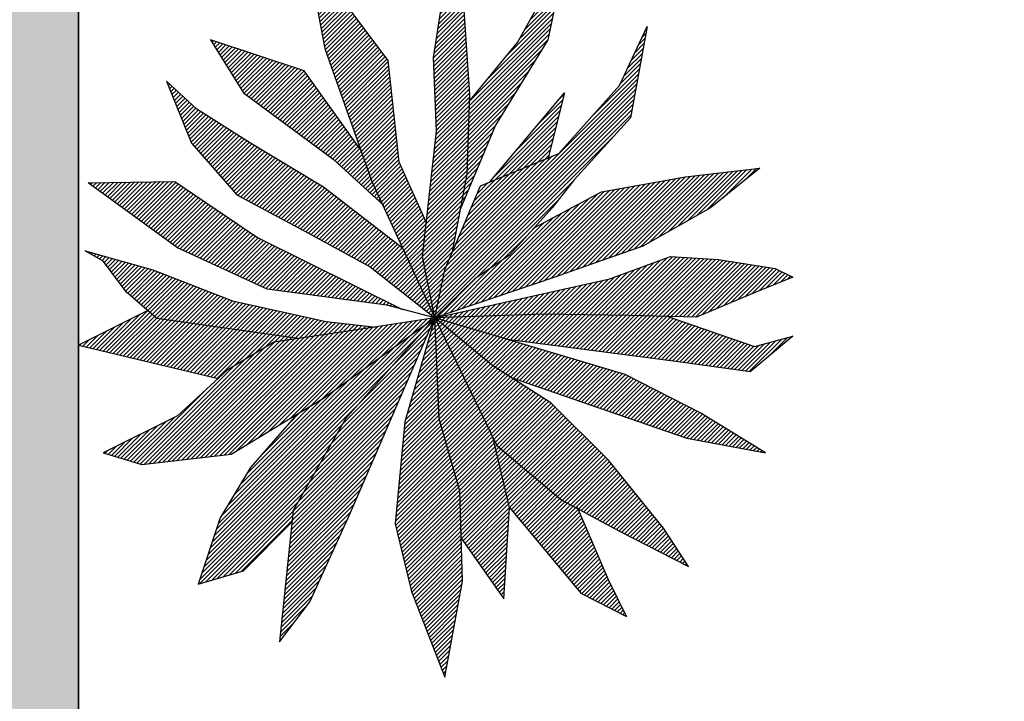
# Model space of a CAD drawing. Units: inches. Extents: x 3008 to 4088, y 1255 to 2137.
# Tile 16 of 30: x 3042 to 3093, y 1909 to 1945. Entities that reach past the tile are written whole.
import ezdxf

# ---------------------------------------------------------------- set-up
doc = ezdxf.new("R2010")
doc.units = ezdxf.units.IN
for name, color, linetype, lineweight in [('C-PROP', 1, 'Continuous', 35), ('C-PROP-PATT', 9, 'Continuous', 13), ('L-PLNT', 3, 'Continuous', 13), ('vfolhas', 114, 'Continuous', 5)]:
    doc.layers.add(name, color=color, linetype=linetype, lineweight=lineweight)
for name, color, linetype in [('vfolha', 72, 'Continuous'), ('vfolha2', 110, 'Continuous'), ('vfolhas2', 102, 'Continuous')]:
    doc.layers.add(name, color=color, linetype=linetype)
pattern_1 = [(45, (-2446.5133113, 50.986076), (-0.004419417382, 0.004419417382), [])]

# ---------------------------------------------------------------- blocks, each defined once
blk = doc.blocks.new('arbusto_PB_verde_grande')
at = {"layer": 'vfolha2'}
h = blk.add_hatch(dxfattribs=at)
h.set_pattern_fill('ANSI31', color=256, scale=0.05, style=0)
h.set_pattern_definition(pattern_1)
h.paths.add_polyline_path([(0.0294, 0.3565), (0.0003, 0.0905), (0.0263, -0.0393), (0.047, 0.0623), (0.0619, 0.0973), (0.0937, 0.2657), (0.0996, 0.4347), (0.0879, 0.6131), (0.0645, 0.7227), (0.0499, 0.6851), (0.0236, 0.5129)])
h.paths.add_polyline_path([(0.3011, 0.4379), (0.1423, 0.2487), (0.2669, 0.3002)])
h.paths.add_polyline_path([(0.38, 0.2282), (0.237, 0.1519), (0.1843, 0.0936), (0.1112, 0.0436), (0.0263, -0.0393), (0.2806, 0.0467), (0.3683, 0.078), (0.4676, 0.1124), (0.6107, 0.1938), (0.7159, 0.2782), (0.5581, 0.2595)])
h.paths.add_polyline_path([(0.561, -0.2944), (0.7275, -0.3257), (0.5902, -0.2412), (0.4296, -0.1598), (0.0263, -0.0393), (0.1492, -0.1411), (0.1884, -0.166), (0.415, -0.2444)])
h.paths.add_polyline_path([(-0.2743, -0.4478), (-0.3035, -0.7263), (-0.2392, -0.6417), (-0.1546, -0.4572), (0.0263, -0.0393), (-0.1633, -0.2538)])
h.paths.add_polyline_path([(-0.5196, -0.2474), (-0.6774, -0.3257), (-0.5956, -0.3507), (-0.4057, -0.3288), (-0.2101, -0.21), (0.0263, -0.0393), (-0.1487, -0.0659), (-0.3152, -0.091), (-0.4145, -0.1505)])
h.paths.add_polyline_path([(-0.5255, 0.2501), (-0.7095, 0.247), (-0.5196, 0.1093), (-0.3298, 0.0217), (-0.0757, -0.0128), (-0.0423, -0.0215), (-0.3502, 0.1312)])
h = blk.add_hatch(dxfattribs=at)
h.set_pattern_fill('ANSI31', color=256, scale=0.05, style=0)
h.set_pattern_definition(pattern_1)
h.paths.add_polyline_path([(-0.1896, 0.297), (-0.0855, 0.2019), (-0.1078, 0.2501), (-0.132, 0.3187), (-0.251, 0.4848), (-0.4495, 0.5505), (-0.3795, 0.4379)])
h.paths.add_polyline_path([(0.0791, -0.4071), (0.0821, -0.5063), (0.1726, -0.6355), (0.1843, -0.4415), (0.149, -0.2918), (0.0263, -0.0393), (0.0353, -0.2538)])
at = {"layer": 'vfolhas'}
h = blk.add_hatch(dxfattribs=at)
h.set_pattern_fill('ANSI31', color=256, scale=0.05, style=0)
h.set_pattern_definition(pattern_1)
h.paths.add_polyline_path([(-0.0728, 0.5067), (-0.1808, 0.6506), (-0.2334, 0.6725), (-0.2071, 0.5318), (-0.1078, 0.2501), (0.0263, -0.0393), (0.0003, 0.0905), (0.0082, 0.1624), (-0.0494, 0.2908)])
h.paths.add_polyline_path([(0.099, 0.4193), (0.0937, 0.2657), (0.0791, 0.1881), (0.1551, 0.369), (0.2661, 0.5505), (0.2836, 0.635), (0.2485, 0.6882), (0.2514, 0.635), (0.2018, 0.5443)])
h.paths.add_polyline_path([(0.1229, 0.2407), (0.047, 0.0623), (0.0263, -0.0393), (0.1112, 0.0436), (0.1843, 0.0936), (0.2748, 0.1938), (0.3215, 0.2532), (0.4413, 0.3847), (0.4763, 0.5787), (0.4179, 0.4535), (0.2894, 0.3095)])
h.paths.add_polyline_path([(0.5815, -0.0378), (0.7071, 0.0154), (0.7859, 0.0467), (0.748, 0.0655), (0.6282, 0.0842), (0.526, 0.0905), (0.3974, 0.0436), (0.0263, -0.0393), (0.2573, -0.0315), (0.4383, -0.0347)])
h.paths.add_polyline_path([(0.5202, -0.0365), (0.4383, -0.0347), (0.2573, -0.0315), (0.0263, -0.0393), (0.1796, -0.0852), (0.5377, -0.1317), (0.6954, -0.1536), (0.7859, -0.0785), (0.7041, -0.1004)])
h.paths.add_polyline_path([(0.2719, -0.2193), (0.1492, -0.1411), (0.0263, -0.0393), (0.1579, -0.3101), (0.2952, -0.4258), (0.4179, -0.4916), (0.564, -0.5667), (0.5114, -0.4853), (0.3946, -0.3414)])
h.paths.add_polyline_path([(-0.0582, -0.4759), (-0.0231, -0.6198), (0.047, -0.8013), (0.0849, -0.5979), (0.0791, -0.4071), (0.0353, -0.2538), (0.0263, -0.0393), (-0.0377, -0.26)])
h.paths.add_polyline_path([(-0.2422, 0.1405), (-0.1107, 0.0686), (0.0263, -0.0393), (-0.0423, 0.1087), (-0.2101, 0.2376), (-0.3649, 0.3314), (-0.4787, 0.4034), (-0.543, 0.4629), (-0.4904, 0.3314), (-0.3941, 0.2219)])
h = blk.add_hatch(dxfattribs=at)
h.set_pattern_fill('ANSI31', color=256, scale=0.05, style=0)
h.set_pattern_definition(pattern_1)
h.paths.add_polyline_path([(-0.5722, 0.0623), (-0.7153, 0.103), (-0.6774, 0.0811), (-0.6277, 0.0154), (-0.5635, -0.041), (-0.2646, -0.0834), (-0.1487, -0.0659), (-0.1015, -0.0588), (-0.2042, -0.0472), (-0.4028, -0.0034)])
h.paths.add_polyline_path([(-0.5635, -0.041), (-0.5828, -0.024), (-0.7299, -0.0973), (-0.4334, -0.1679), (-0.4145, -0.1505), (-0.3152, -0.091), (-0.2646, -0.0834)])
h.paths.add_polyline_path([(-0.2769, -0.4727), (-0.2743, -0.4478), (-0.1633, -0.2538), (0.0263, -0.0393), (-0.2101, -0.21), (-0.2672, -0.2447), (-0.3649, -0.357), (-0.4291, -0.4634), (-0.4759, -0.6043), (-0.3795, -0.576)])
h = blk.add_hatch(dxfattribs=at)
h.set_pattern_fill('ANSI31', color=256, scale=0.05, style=0)
h.set_pattern_definition(pattern_1)
h.paths.add_polyline_path([(0.3361, -0.623), (0.4325, -0.6731), (0.3946, -0.5948), (0.3303, -0.4446), (0.2952, -0.4258), (0.1579, -0.3101), (0.149, -0.2918), (0.1843, -0.4415)])
at = {"layer": 'vfolha'}
for p, q in [((0.0263, -0.0393), (-0.1487, -0.0659)), ((0.0263, -0.0393), (-0.0377, -0.26)), ((0.0353, -0.2538), (0.0263, -0.0393)), ((0.5202, -0.0365), (0.7041, -0.1004)), ((0.7859, -0.0785), (0.6954, -0.1536)), ((0.7041, -0.1004), (0.7859, -0.0785)), ((0.5377, -0.1317), (0.1796, -0.0852)), ((0.6954, -0.1536), (0.5377, -0.1317)), ((0.3946, -0.3414), (0.2719, -0.2193)), ((-0.2672, -0.2447), (-0.3649, -0.357)), ((-0.0377, -0.26), (-0.0582, -0.4759)), ((0.0791, -0.4071), (0.0353, -0.2538)), ((0.1579, -0.3101), (0.2952, -0.4258)), ((0.5114, -0.4853), (0.3946, -0.3414)), ((0.0849, -0.5979), (0.0791, -0.4071)), ((0.2952, -0.4258), (0.4179, -0.4916)), ((0.4179, -0.4916), (0.564, -0.5667)), ((0.564, -0.5667), (0.5114, -0.4853)), ((0.047, -0.8013), (0.0849, -0.5979)), ((-0.0231, -0.6198), (0.047, -0.8013))]:
    blk.add_line(p, q, dxfattribs=at)
at = {"layer": 'vfolha2'}
for p, q in [((0.0499, 0.6851), (0.0645, 0.7227)), ((0.0645, 0.7227), (0.0879, 0.6131)), ((0.0236, 0.5129), (0.0499, 0.6851)), ((0.0879, 0.6131), (0.0996, 0.4347)), ((-0.4495, 0.5505), (-0.3795, 0.4379)), ((-0.251, 0.4848), (-0.4495, 0.5505)), ((0.0294, 0.3565), (0.0236, 0.5129)), ((-0.132, 0.3187), (-0.251, 0.4848)), ((-0.3795, 0.4379), (-0.1896, 0.297)), ((0.0996, 0.4347), (0.0937, 0.2657)), ((0.1434, 0.2501), (0.3011, 0.4379)), ((0.3011, 0.4379), (0.2661, 0.297)), ((0.0003, 0.0905), (0.0294, 0.3565)), ((-0.1896, 0.297), (-0.0822, 0.1989)), ((0.5581, 0.2595), (0.7159, 0.2782)), ((0.7159, 0.2782), (0.6107, 0.1938)), ((0.38, 0.2282), (0.5581, 0.2595)), ((-0.7095, 0.247), (-0.5255, 0.2501)), ((-0.5196, 0.1093), (-0.7095, 0.247)), ((-0.5255, 0.2501), (-0.3502, 0.1312)), ((0.237, 0.1519), (0.38, 0.2282)), ((0.6107, 0.1938), (0.4676, 0.1124)), ((-0.3502, 0.1312), (-0.0423, -0.0215)), ((-0.3298, 0.0217), (-0.5196, 0.1093)), ((0.0263, -0.0393), (0.0003, 0.0905)), ((0.3683, 0.078), (0.2806, 0.0467)), ((0.2806, 0.0467), (0.0263, -0.0393)), ((-0.0757, -0.0128), (-0.3298, 0.0217)), ((-0.2101, -0.21), (0.0263, -0.0393)), ((0.0263, -0.0393), (-0.1633, -0.2538)), ((-0.1546, -0.4572), (0.0263, -0.0393)), ((0.4296, -0.1598), (0.0263, -0.0393)), ((0.0263, -0.0393), (0.1579, -0.3101)), ((-0.1487, -0.0659), (-0.3152, -0.091)), ((-0.3152, -0.091), (-0.4145, -0.1505)), ((-0.4145, -0.1505), (-0.5196, -0.2474)), ((0.1884, -0.166), (0.415, -0.2444)), ((0.5902, -0.2412), (0.4296, -0.1598)), ((-0.4057, -0.3288), (-0.2101, -0.21)), ((-0.5196, -0.2474), (-0.6774, -0.3257)), ((0.415, -0.2444), (0.561, -0.2944)), ((0.7275, -0.3257), (0.5902, -0.2412)), ((-0.1633, -0.2538), (-0.2743, -0.4478)), ((0.1843, -0.4415), (0.149, -0.2918)), ((0.561, -0.2944), (0.7275, -0.3257)), ((-0.6774, -0.3257), (-0.5956, -0.3507)), ((-0.5956, -0.3507), (-0.4057, -0.3288)), ((-0.2743, -0.4478), (-0.3035, -0.7263)), ((0.1726, -0.6355), (0.1843, -0.4415)), ((0.0821, -0.5063), (0.1726, -0.6355)), ((-0.3035, -0.7263), (-0.2392, -0.6417))]:
    blk.add_line(p, q, dxfattribs=at)
at = {"layer": 'vfolhas2'}
for p, q in [((-0.2334, 0.6725), (-0.2071, 0.5318)), ((-0.1808, 0.6506), (-0.2334, 0.6725)), ((0.2514, 0.635), (0.2485, 0.6882)), ((0.2485, 0.6882), (0.2836, 0.635)), ((-0.0728, 0.5067), (-0.1808, 0.6506)), ((0.2018, 0.5443), (0.2514, 0.635)), ((0.2836, 0.635), (0.2661, 0.5505)), ((0.4179, 0.4535), (0.4763, 0.5787)), ((0.4763, 0.5787), (0.4413, 0.3847)), ((0.099, 0.4193), (0.2018, 0.5443)), ((0.2661, 0.5505), (0.1551, 0.369)), ((-0.2071, 0.5318), (-0.1078, 0.2501)), ((-0.0494, 0.2908), (-0.0728, 0.5067)), ((-0.543, 0.4629), (-0.4904, 0.3314)), ((-0.4787, 0.4034), (-0.543, 0.4629)), ((0.2894, 0.3095), (0.4179, 0.4535)), ((-0.3649, 0.3314), (-0.4787, 0.4034)), ((0.4413, 0.3847), (0.3215, 0.2532)), ((0.1551, 0.369), (0.078, 0.1855)), ((-0.4904, 0.3314), (-0.3941, 0.2219)), ((-0.2101, 0.2376), (-0.3649, 0.3314)), ((0.1229, 0.2407), (0.2894, 0.3095)), ((0.0082, 0.1624), (-0.0494, 0.2908)), ((0.0937, 0.2657), (0.0619, 0.0973)), ((0.3215, 0.2532), (0.2748, 0.1938)), ((-0.0423, 0.1087), (-0.2101, 0.2376)), ((-0.1078, 0.2501), (0.0263, -0.0393)), ((0.047, 0.0623), (0.1229, 0.2407)), ((-0.3941, 0.2219), (-0.2422, 0.1405)), ((0.2748, 0.1938), (0.1843, 0.0936)), ((-0.2422, 0.1405), (-0.1107, 0.0686)), ((0.4676, 0.1124), (0.3683, 0.078)), ((-0.6774, 0.0811), (-0.7153, 0.103)), ((-0.7153, 0.103), (-0.5722, 0.0623)), ((0.1843, 0.0936), (0.1112, 0.0436)), ((0.3974, 0.0436), (0.526, 0.0905)), ((0.526, 0.0905), (0.6282, 0.0842)), ((0.6282, 0.0842), (0.748, 0.0655)), ((-0.6277, 0.0154), (-0.6774, 0.0811)), ((-0.1107, 0.0686), (0.0263, -0.0393)), ((0.748, 0.0655), (0.7859, 0.0467)), ((-0.5722, 0.0623), (-0.4028, -0.0034)), ((0.0263, -0.0393), (0.047, 0.0623)), ((0.0263, -0.0393), (0.3974, 0.0436)), ((0.1112, 0.0436), (0.0263, -0.0393)), ((0.7859, 0.0467), (0.7071, 0.0154)), ((-0.5635, -0.041), (-0.6277, 0.0154)), ((0.7071, 0.0154), (0.5815, -0.0378)), ((-0.4028, -0.0034), (-0.2042, -0.0472)), ((0.0263, -0.0393), (-0.0757, -0.0128)), ((-0.5828, -0.024), (-0.7299, -0.0973)), ((-0.2646, -0.0834), (-0.5635, -0.041)), ((0.2573, -0.0315), (0.0263, -0.0393)), ((0.1492, -0.1411), (0.0263, -0.0393)), ((0.4383, -0.0347), (0.2573, -0.0315)), ((0.5815, -0.0378), (0.4383, -0.0347)), ((-0.2042, -0.0472), (-0.0983, -0.0591)), ((-0.7299, -0.0973), (-0.4334, -0.1679)), ((0.2719, -0.2193), (0.1492, -0.1411)), ((-0.3649, -0.357), (-0.4291, -0.4634)), ((-0.2392, -0.6417), (-0.1546, -0.4572)), ((0.1843, -0.4415), (0.3361, -0.623)), ((0.3946, -0.5948), (0.329, -0.4417)), ((-0.4291, -0.4634), (-0.4759, -0.6043)), ((-0.3795, -0.576), (-0.2769, -0.4727)), ((-0.0582, -0.4759), (-0.0231, -0.6198)), ((-0.4759, -0.6043), (-0.3795, -0.576)), ((0.4325, -0.6731), (0.3946, -0.5948)), ((0.3361, -0.623), (0.4325, -0.6731))]:
    blk.add_line(p, q, dxfattribs=at)

msp = doc.modelspace()

# ---------------------------------------------------------------- hatches: boundary and pattern name
at = {"layer": 'C-PROP-PATT'}
h = msp.add_hatch(color=256, dxfattribs=at)
h.dxf.hatch_style = 1
h.paths.add_polyline_path([(3519.666, 2003.966), (3039.666, 2003.966), (3039.666, 1343.966), (3051.666, 1343.966), (3051.666, 1348.966), (3044.666, 1348.966), (3044.666, 1998.966), (3514.666, 1998.966), (3514.666, 1348.966), (3219.666, 1348.966), (3219.666, 1343.966), (3519.666, 1343.966)])

# ---------------------------------------------------------------- linework, layer by layer
at = {"layer": 'C-PROP'}
msp.add_line((3044.666, 1348.966), (3044.666, 1998.966), dxfattribs=at)

# ---------------------------------------------------------------- block references
at = {"layer": 'L-PLNT', "xscale": 24.60366729364114, "yscale": 24.60366729364114, "zscale": 24.60366729364114}
msp.add_blockref('arbusto_PB_verde_grande', (3062.624, 1930.394), dxfattribs=at)

doc.saveas('drawing.dxf')
